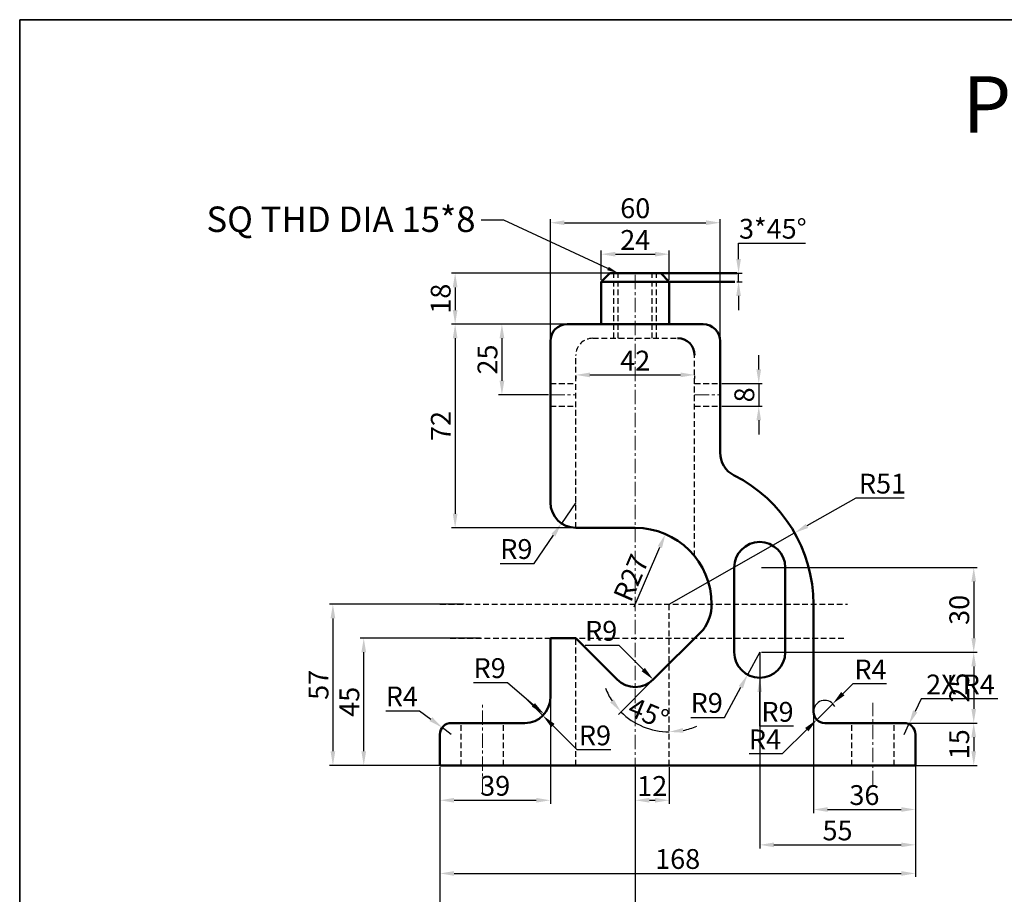
# Model space of a CAD drawing. Units: millimetres. Extents: x -39 to 854, y -107 to 478.
# Tile 2 of 4: x -39 to 309, y 169 to 478. Entities that reach past the tile are written whole.
import ezdxf
from ezdxf import colors
from ezdxf.entities.mleader import LeaderData, LeaderLine
from ezdxf.math import Vec2, Vec3

# ---------------------------------------------------------------- set-up
doc = ezdxf.new("R2010")
doc.units = ezdxf.units.MM
doc.header["$LTSCALE"] = 0.4
doc.linetypes.add('CENTER', pattern=[50.8, 31.75, -6.35, 6.35, -6.35])
doc.linetypes.add('DASHED', pattern=[19.05, 12.7, -6.35])
for name, color, linetype, lineweight in [('M-CNTR', 1, 'CENTER', 18), ('M-DIMS', 2, 'Continuous', 25), ('M-HIDN', 6, 'DASHED', 25), ('M-OUTL', 7, 'Continuous', 50), ('M-TEXT', 3, 'Continuous', 25), ('M-TTLB', 7, 'Continuous', 35)]:
    doc.layers.add(name, color=color, linetype=linetype, lineweight=lineweight)
doc.styles.get("Standard").update_dxf_attribs({"font": 'arial.ttf'})
doc.dimstyles.new('ISO-25', dxfattribs={"dimtxt": 7, "dimasz": 5, "dimexe": 1.25, "dimexo": 0.625, "dimtad": 1, "dimtoh": 1, "dimtxsty": 'Standard', "dimcen": 2.5, "dimadec": 0, "dimazin": 0, "dimtfac": 1, "dimtmove": 0, "dimatfit": 3, "dimfxl": 1, "dimarcsym": 0})

# ---------------------------------------------------------------- blocks, each defined once
blk = doc.blocks.new('*D14')
at = {"layer": 'Defpoints', "color": 0, "ltscale": 0.4, "transparency": 16777216}
for p in [(109.61, 214.19), (277.61, 214.19), (277.61, 176.03)]:
    blk.add_point(p, dxfattribs=at)
at = {"layer": 'M-DIMS', "color": 0, "lineweight": -2, "ltscale": 0.4, "transparency": 16777216}
for p, q in [((109.61, 213.56), (109.61, 174.78)), ((277.61, 213.56), (277.61, 174.78)), ((114.61, 176.03), (272.61, 176.03))]:
    blk.add_line(p, q, dxfattribs=at)
at = {"layer": 'M-DIMS', "color": 0, "ltscale": 0.4, "transparency": 16777216}
for points in [[(114.61, 176.86), (114.61, 175.2), (109.61, 176.03)], [(272.61, 176.86), (272.61, 175.2), (277.61, 176.03)]]:
    blk.add_solid(points, dxfattribs=at)
at = {"layer": 'M-DIMS', "color": 0, "ltscale": 0.4, "transparency": 16777216, "insert": (193.61, 180.23), "char_height": 7, "attachment_point": 5}
blk.add_mtext('168', dxfattribs=at)
blk = doc.blocks.new('*D15')
at = {"layer": 'Defpoints', "color": 0, "ltscale": 0.4, "transparency": 16777216}
for p in [(148.61, 238.19), (109.61, 214.19), (148.61, 201.89)]:
    blk.add_point(p, dxfattribs=at)
at = {"layer": 'M-DIMS', "color": 0, "lineweight": -2, "ltscale": 0.4, "transparency": 16777216}
for p, q in [((148.61, 237.56), (148.61, 200.64)), ((109.61, 213.56), (109.61, 200.64)), ((114.61, 201.89), (143.61, 201.89))]:
    blk.add_line(p, q, dxfattribs=at)
at = {"layer": 'M-DIMS', "color": 0, "ltscale": 0.4, "transparency": 16777216}
for points in [[(114.61, 202.73), (114.61, 201.06), (109.61, 201.89)], [(143.61, 202.73), (143.61, 201.06), (148.61, 201.89)]]:
    blk.add_solid(points, dxfattribs=at)
at = {"layer": 'M-DIMS', "color": 0, "ltscale": 0.4, "transparency": 16777216, "insert": (129.11, 206.1), "char_height": 7, "attachment_point": 5}
blk.add_mtext('39', dxfattribs=at)
blk = doc.blocks.new('*D16')
at = {"layer": 'Defpoints', "color": 0, "ltscale": 0.4, "transparency": 16777216}
for p in [(190.61, 214.19), (178.61, 207.01), (190.61, 201.89)]:
    blk.add_point(p, dxfattribs=at)
at = {"layer": 'M-DIMS', "color": 0, "lineweight": -2, "ltscale": 0.4, "transparency": 16777216}
for p, q in [((190.61, 213.56), (190.61, 200.64)), ((178.61, 206.38), (178.61, 200.64)), ((183.61, 201.89), (185.61, 201.89))]:
    blk.add_line(p, q, dxfattribs=at)
at = {"layer": 'M-DIMS', "color": 0, "ltscale": 0.4, "transparency": 16777216}
for points in [[(183.61, 202.73), (183.61, 201.06), (178.61, 201.89)], [(185.61, 202.73), (185.61, 201.06), (190.61, 201.89)]]:
    blk.add_solid(points, dxfattribs=at)
at = {"layer": 'M-DIMS', "color": 0, "ltscale": 0.4, "transparency": 16777216, "insert": (184.61, 206.03), "char_height": 7, "attachment_point": 5}
blk.add_mtext('12', dxfattribs=at)
blk = doc.blocks.new('*D17')
at = {"layer": 'Defpoints', "color": 0, "ltscale": 0.4, "transparency": 16777216}
for p in [(222.61, 254.19), (277.61, 200.76), (277.61, 186.13)]:
    blk.add_point(p, dxfattribs=at)
at = {"layer": 'M-DIMS', "color": 0, "lineweight": -2, "ltscale": 0.4, "transparency": 16777216}
for p, q in [((222.61, 253.56), (222.61, 184.88)), ((277.61, 200.14), (277.61, 184.88)), ((227.61, 186.13), (272.61, 186.13))]:
    blk.add_line(p, q, dxfattribs=at)
at = {"layer": 'M-DIMS', "color": 0, "ltscale": 0.4, "transparency": 16777216}
for points in [[(227.61, 186.96), (227.61, 185.3), (222.61, 186.13)], [(272.61, 186.96), (272.61, 185.3), (277.61, 186.13)]]:
    blk.add_solid(points, dxfattribs=at)
at = {"layer": 'M-DIMS', "color": 0, "ltscale": 0.4, "transparency": 16777216, "insert": (250.11, 190.32), "char_height": 7, "attachment_point": 5}
blk.add_mtext('55', dxfattribs=at)
blk = doc.blocks.new('*D18')
at = {"layer": 'Defpoints', "color": 0, "ltscale": 0.4, "transparency": 16777216}
for p in [(241.61, 238.74), (277.61, 219.69), (277.61, 198.62)]:
    blk.add_point(p, dxfattribs=at)
at = {"layer": 'M-DIMS', "color": 0, "lineweight": -2, "ltscale": 0.4, "transparency": 16777216}
for p, q in [((241.61, 238.11), (241.61, 197.37)), ((277.61, 219.06), (277.61, 197.37)), ((246.61, 198.62), (272.61, 198.62))]:
    blk.add_line(p, q, dxfattribs=at)
at = {"layer": 'M-DIMS', "color": 0, "ltscale": 0.4, "transparency": 16777216}
for points in [[(246.61, 199.45), (246.61, 197.79), (241.61, 198.62)], [(272.61, 199.45), (272.61, 197.79), (277.61, 198.62)]]:
    blk.add_solid(points, dxfattribs=at)
at = {"layer": 'M-DIMS', "color": 0, "ltscale": 0.4, "transparency": 16777216, "insert": (259.61, 202.82), "char_height": 7, "attachment_point": 5}
blk.add_mtext('36', dxfattribs=at)
blk = doc.blocks.new('*D19')
at = {"layer": 'Defpoints', "color": 0, "ltscale": 0.4, "transparency": 16777216}
for p in [(270.11, 229.19), (270.11, 214.19), (298.24, 214.19)]:
    blk.add_point(p, dxfattribs=at)
at = {"layer": 'M-DIMS', "color": 0, "lineweight": -2, "ltscale": 0.4, "transparency": 16777216}
for p, q in [((270.73, 229.19), (299.49, 229.19)), ((298.24, 224.19), (298.24, 219.19)), ((270.73, 214.19), (299.49, 214.19))]:
    blk.add_line(p, q, dxfattribs=at)
at = {"layer": 'M-DIMS', "color": 0, "ltscale": 0.4, "transparency": 16777216}
for points in [[(297.41, 224.19), (299.07, 224.19), (298.24, 229.19)], [(297.41, 219.19), (299.07, 219.19), (298.24, 214.19)]]:
    blk.add_solid(points, dxfattribs=at)
at = {"layer": 'M-DIMS', "color": 0, "ltscale": 0.4, "transparency": 16777216, "insert": (294.04, 221.69), "char_height": 7, "attachment_point": 5, "rotation": 90}
blk.add_mtext('15', dxfattribs=at)
blk = doc.blocks.new('*D20')
at = {"layer": 'Defpoints', "color": 0, "ltscale": 0.4, "transparency": 16777216}
for p in [(222.61, 254.19), (270.11, 229.19), (298.24, 229.19)]:
    blk.add_point(p, dxfattribs=at)
at = {"layer": 'M-DIMS', "color": 0, "lineweight": -2, "ltscale": 0.4, "transparency": 16777216}
for p, q in [((223.23, 254.19), (299.49, 254.19)), ((298.24, 249.19), (298.24, 234.19)), ((270.73, 229.19), (299.49, 229.19))]:
    blk.add_line(p, q, dxfattribs=at)
at = {"layer": 'M-DIMS', "color": 0, "ltscale": 0.4, "transparency": 16777216}
for points in [[(297.41, 249.19), (299.07, 249.19), (298.24, 254.19)], [(297.41, 234.19), (299.07, 234.19), (298.24, 229.19)]]:
    blk.add_solid(points, dxfattribs=at)
at = {"layer": 'M-DIMS', "color": 0, "ltscale": 0.4, "transparency": 16777216, "insert": (294.04, 241.69), "char_height": 7, "attachment_point": 5, "rotation": 90}
blk.add_mtext('25', dxfattribs=at)
blk = doc.blocks.new('*D21')
at = {"layer": 'Defpoints', "color": 0, "ltscale": 0.4, "transparency": 16777216}
for p in [(222.61, 284.19), (261.36, 254.19), (298.24, 254.19)]:
    blk.add_point(p, dxfattribs=at)
at = {"layer": 'M-DIMS', "color": 0, "lineweight": -2, "ltscale": 0.4, "transparency": 16777216}
for p, q in [((223.23, 284.19), (299.49, 284.19)), ((298.24, 279.19), (298.24, 259.19)), ((261.99, 254.19), (299.49, 254.19))]:
    blk.add_line(p, q, dxfattribs=at)
at = {"layer": 'M-DIMS', "color": 0, "ltscale": 0.4, "transparency": 16777216}
for points in [[(297.41, 279.19), (299.07, 279.19), (298.24, 284.19)], [(297.41, 259.19), (299.07, 259.19), (298.24, 254.19)]]:
    blk.add_solid(points, dxfattribs=at)
at = {"layer": 'M-DIMS', "color": 0, "ltscale": 0.4, "transparency": 16777216, "insert": (294.04, 269.19), "char_height": 7, "attachment_point": 5, "rotation": 90}
blk.add_mtext('30', dxfattribs=at)
blk = doc.blocks.new('*D22')
at = {"layer": 'Defpoints', "color": 0, "ltscale": 0.4, "transparency": 16777216}
for p in [(234.94, 296.4), (190.61, 271.19)]:
    blk.add_point(p, dxfattribs=at)
at = {"layer": 'M-DIMS', "color": 0, "lineweight": -2, "ltscale": 0.4, "transparency": 16777216}
for p, q in [((256.59, 308.71), (239.29, 298.87)), ((273.69, 308.71), (256.59, 308.71)), ((190.61, 271.19), (234.94, 296.4))]:
    blk.add_line(p, q, dxfattribs=at)
at = {"layer": 'M-DIMS', "color": 0, "ltscale": 0.4, "transparency": 16777216}
blk.add_solid([(238.87, 299.59), (239.7, 298.15), (234.94, 296.4)], dxfattribs=at)
at = {"layer": 'M-DIMS', "color": 0, "ltscale": 0.4, "transparency": 16777216, "insert": (266, 312.91), "char_height": 7, "attachment_point": 5}
blk.add_mtext('R51', dxfattribs=at)
blk = doc.blocks.new('*D23')
at = {"layer": 'Defpoints', "color": 0, "ltscale": 0.4, "transparency": 16777216}
for p in [(222.61, 254.19), (218.32, 246.28)]:
    blk.add_point(p, dxfattribs=at)
at = {"layer": 'M-DIMS', "color": 0, "lineweight": -2, "ltscale": 0.4, "transparency": 16777216}
for p, q in [((222.61, 254.19), (218.32, 246.28)), ((210.14, 231.2), (215.93, 241.88)), ((198.22, 231.2), (210.14, 231.2))]:
    blk.add_line(p, q, dxfattribs=at)
at = {"layer": 'M-DIMS', "color": 0, "ltscale": 0.4, "transparency": 16777216}
blk.add_solid([(215.2, 242.28), (216.67, 241.48), (218.32, 246.28)], dxfattribs=at)
at = {"layer": 'M-DIMS', "color": 0, "ltscale": 0.4, "transparency": 16777216, "insert": (203.87, 235.4), "char_height": 7, "attachment_point": 5}
blk.add_mtext('R9', dxfattribs=at)
blk = doc.blocks.new('*D24')
at = {"layer": 'Defpoints', "color": 0, "ltscale": 0.4, "transparency": 16777216}
for p in [(110.4, 227.58), (113.61, 225.19)]:
    blk.add_point(p, dxfattribs=at)
at = {"layer": 'M-DIMS', "color": 0, "lineweight": -2, "ltscale": 0.4, "transparency": 16777216}
for p, q in [((90.5, 233.56), (102.39, 233.56)), ((102.39, 233.56), (106.4, 230.57)), ((113.61, 225.19), (110.4, 227.58))]:
    blk.add_line(p, q, dxfattribs=at)
at = {"layer": 'M-DIMS', "color": 0, "ltscale": 0.4, "transparency": 16777216}
blk.add_solid([(106.89, 231.24), (105.9, 229.9), (110.4, 227.58)], dxfattribs=at)
at = {"layer": 'M-DIMS', "color": 0, "ltscale": 0.4, "transparency": 16777216, "insert": (96.13, 237.69), "char_height": 7, "attachment_point": 5}
blk.add_mtext('R4', dxfattribs=at)
blk = doc.blocks.new('*D25')
at = {"layer": 'Defpoints', "color": 0, "ltscale": 0.4, "transparency": 16777216}
for p in [(157.61, 307.19), (152.53, 299.75)]:
    blk.add_point(p, dxfattribs=at)
at = {"layer": 'M-DIMS', "color": 0, "lineweight": -2, "ltscale": 0.4, "transparency": 16777216}
for p, q in [((157.61, 307.19), (152.53, 299.75)), ((142.86, 285.59), (149.71, 295.63)), ((130.93, 285.59), (142.86, 285.59))]:
    blk.add_line(p, q, dxfattribs=at)
at = {"layer": 'M-DIMS', "color": 0, "ltscale": 0.4, "transparency": 16777216}
blk.add_solid([(149.02, 296.1), (150.4, 295.16), (152.53, 299.75)], dxfattribs=at)
at = {"layer": 'M-DIMS', "color": 0, "ltscale": 0.4, "transparency": 16777216, "insert": (136.59, 289.79), "char_height": 7, "attachment_point": 5}
blk.add_mtext('R9', dxfattribs=at)
blk = doc.blocks.new('*D26')
at = {"layer": 'Defpoints', "color": 0, "ltscale": 0.4, "transparency": 16777216}
for p in [(118.77, 271.19), (71.76, 214.19), (117.11, 214.19)]:
    blk.add_point(p, dxfattribs=at)
at = {"layer": 'M-DIMS', "color": 0, "lineweight": -2, "ltscale": 0.4, "transparency": 16777216}
for p, q in [((118.14, 271.19), (70.51, 271.19)), ((71.76, 266.19), (71.76, 219.19)), ((116.48, 214.19), (70.51, 214.19))]:
    blk.add_line(p, q, dxfattribs=at)
at = {"layer": 'M-DIMS', "color": 0, "ltscale": 0.4, "transparency": 16777216}
for points in [[(70.93, 266.19), (72.6, 266.19), (71.76, 271.19)], [(70.93, 219.19), (72.6, 219.19), (71.76, 214.19)]]:
    blk.add_solid(points, dxfattribs=at)
at = {"layer": 'M-DIMS', "color": 0, "ltscale": 0.4, "transparency": 16777216, "insert": (67.58, 242.69), "char_height": 7, "attachment_point": 5, "rotation": 90}
blk.add_mtext('57', dxfattribs=at)
blk = doc.blocks.new('*D27')
at = {"layer": 'Defpoints', "color": 0, "ltscale": 0.4, "transparency": 16777216}
for p in [(82.66, 259.19), (124.61, 259.19), (124.61, 214.19)]:
    blk.add_point(p, dxfattribs=at)
at = {"layer": 'M-DIMS', "color": 0, "lineweight": -2, "ltscale": 0.4, "transparency": 16777216}
for p, q in [((123.98, 259.19), (81.41, 259.19)), ((82.66, 219.19), (82.66, 254.19)), ((123.98, 214.19), (81.41, 214.19))]:
    blk.add_line(p, q, dxfattribs=at)
at = {"layer": 'M-DIMS', "color": 0, "ltscale": 0.4, "transparency": 16777216}
for points in [[(81.83, 254.19), (83.5, 254.19), (82.66, 259.19)], [(81.83, 219.19), (83.5, 219.19), (82.66, 214.19)]]:
    blk.add_solid(points, dxfattribs=at)
at = {"layer": 'M-DIMS', "color": 0, "ltscale": 0.4, "transparency": 16777216, "insert": (78.48, 236.69), "char_height": 7, "attachment_point": 5, "rotation": 90}
blk.add_mtext('45', dxfattribs=at)
blk = doc.blocks.new('*D28')
at = {"layer": 'Defpoints', "color": 0, "ltscale": 0.4, "transparency": 16777216}
for p in [(190.61, 271.19), (202.61, 262.19), (184.97, 244.55), (178.55, 229.3), (190.61, 214.19)]:
    blk.add_point(p, dxfattribs=at)
at = {"layer": 'M-DIMS', "color": 0, "lineweight": -2, "ltscale": 0.4, "transparency": 16777216}
blk.add_line((184.53, 244.11), (172.67, 232.25), dxfattribs=at)
for start, end in [(201.2009, 213.1005), (225, 270), (281.8995, 293.7991)]:
    blk.add_arc((190.61, 250.19), 24.12, start, end, dxfattribs=at)
at = {"layer": 'M-DIMS', "color": 0, "ltscale": 0.4, "transparency": 16777216}
for points in [[(171.05, 237.54), (169.76, 236.49), (173.55, 233.13)], [(195.67, 225.76), (195.49, 227.42), (190.61, 226.07)]]:
    blk.add_solid(points, dxfattribs=at)
at = {"layer": 'M-DIMS', "color": 0, "ltscale": 0.4, "transparency": 16777216, "insert": (182.98, 231.77), "char_height": 7, "attachment_point": 5, "rotation": 337.5}
blk.add_mtext('45°', dxfattribs=at)
blk = doc.blocks.new('*D29')
at = {"layer": 'Defpoints', "color": 0, "ltscale": 0.4, "transparency": 16777216}
for p in [(178.61, 250.92), (184.97, 244.55)]:
    blk.add_point(p, dxfattribs=at)
at = {"layer": 'M-DIMS', "color": 0, "lineweight": -2, "ltscale": 0.4, "transparency": 16777216}
for p, q in [((160.92, 256.68), (172.84, 256.68)), ((172.84, 256.68), (181.43, 248.09))]:
    blk.add_line(p, q, dxfattribs=at)
at = {"layer": 'M-DIMS', "color": 0, "ltscale": 0.4, "transparency": 16777216}
blk.add_solid([(182.02, 248.68), (180.85, 247.5), (184.97, 244.55)], dxfattribs=at)
at = {"layer": 'M-DIMS', "color": 0, "ltscale": 0.4, "transparency": 16777216, "insert": (166.57, 260.88), "char_height": 7, "attachment_point": 5}
blk.add_mtext('R9', dxfattribs=at)
blk = doc.blocks.new('*D30')
at = {"layer": 'Defpoints', "color": 0, "ltscale": 0.4, "transparency": 16777216}
for p in [(166.61, 370.19), (114.96, 298.19), (168.11, 298.19)]:
    blk.add_point(p, dxfattribs=at)
at = {"layer": 'M-DIMS', "color": 0, "lineweight": -2, "ltscale": 0.4, "transparency": 16777216}
for p, q in [((165.98, 370.19), (113.71, 370.19)), ((114.96, 365.19), (114.96, 303.19)), ((167.48, 298.19), (113.71, 298.19))]:
    blk.add_line(p, q, dxfattribs=at)
at = {"layer": 'M-DIMS', "color": 0, "ltscale": 0.4, "transparency": 16777216}
for points in [[(114.13, 365.19), (115.8, 365.19), (114.96, 370.19)], [(114.13, 303.19), (115.8, 303.19), (114.96, 298.19)]]:
    blk.add_solid(points, dxfattribs=at)
at = {"layer": 'M-DIMS', "color": 0, "ltscale": 0.4, "transparency": 16777216, "insert": (110.82, 334.19), "char_height": 7, "attachment_point": 5, "rotation": 90}
blk.add_mtext('72', dxfattribs=at)
blk = doc.blocks.new('*D31')
at = {"layer": 'Defpoints', "color": 0, "ltscale": 0.4, "transparency": 16777216}
for p in [(178.61, 388.19), (114.96, 370.19), (178.61, 370.19)]:
    blk.add_point(p, dxfattribs=at)
at = {"layer": 'M-DIMS', "color": 0, "lineweight": -2, "ltscale": 0.4, "transparency": 16777216}
for p, q in [((177.98, 388.19), (113.71, 388.19)), ((114.96, 383.19), (114.96, 375.19)), ((177.98, 370.19), (113.71, 370.19))]:
    blk.add_line(p, q, dxfattribs=at)
at = {"layer": 'M-DIMS', "color": 0, "ltscale": 0.4, "transparency": 16777216}
for points in [[(114.13, 383.19), (115.8, 383.19), (114.96, 388.19)], [(114.13, 375.19), (115.8, 375.19), (114.96, 370.19)]]:
    blk.add_solid(points, dxfattribs=at)
at = {"layer": 'M-DIMS', "color": 0, "ltscale": 0.4, "transparency": 16777216, "insert": (110.76, 379.19), "char_height": 7, "attachment_point": 5, "rotation": 90}
blk.add_mtext('18', dxfattribs=at)
blk = doc.blocks.new('*D32')
at = {"layer": 'Defpoints', "color": 0, "ltscale": 0.4, "transparency": 16777216}
for p in [(139.85, 370.19), (131.5, 345.19), (148.61, 345.19)]:
    blk.add_point(p, dxfattribs=at)
at = {"layer": 'M-DIMS', "color": 0, "lineweight": -2, "ltscale": 0.4, "transparency": 16777216}
for p, q in [((139.22, 370.19), (130.25, 370.19)), ((131.5, 365.19), (131.5, 350.19)), ((147.98, 345.19), (130.25, 345.19))]:
    blk.add_line(p, q, dxfattribs=at)
at = {"layer": 'M-DIMS', "color": 0, "ltscale": 0.4, "transparency": 16777216}
for points in [[(130.67, 365.19), (132.34, 365.19), (131.5, 370.19)], [(130.67, 350.19), (132.34, 350.19), (131.5, 345.19)]]:
    blk.add_solid(points, dxfattribs=at)
at = {"layer": 'M-DIMS', "color": 0, "ltscale": 0.4, "transparency": 16777216, "insert": (127.3, 357.69), "char_height": 7, "attachment_point": 5, "rotation": 90}
blk.add_mtext('25', dxfattribs=at)
blk = doc.blocks.new('*D33')
at = {"layer": 'Defpoints', "color": 0, "ltscale": 0.4, "transparency": 16777216}
for p in [(208.61, 349.19), (208.61, 341.19), (222.27, 341.19)]:
    blk.add_point(p, dxfattribs=at)
at = {"layer": 'M-DIMS', "color": 0, "lineweight": -2, "ltscale": 0.4, "transparency": 16777216}
for p, q in [((222.27, 354.19), (222.27, 359.19)), ((209.23, 349.19), (223.52, 349.19)), ((222.27, 349.19), (222.27, 341.19)), ((209.23, 341.19), (223.52, 341.19)), ((222.27, 336.19), (222.27, 331.19))]:
    blk.add_line(p, q, dxfattribs=at)
at = {"layer": 'M-DIMS', "color": 0, "ltscale": 0.4, "transparency": 16777216}
for points in [[(221.44, 354.19), (223.1, 354.19), (222.27, 349.19)], [(221.44, 336.19), (223.1, 336.19), (222.27, 341.19)]]:
    blk.add_solid(points, dxfattribs=at)
at = {"layer": 'M-DIMS', "color": 0, "ltscale": 0.4, "transparency": 16777216, "insert": (218.07, 345.19), "char_height": 7, "attachment_point": 5, "rotation": 90}
blk.add_mtext('8', dxfattribs=at)
blk = doc.blocks.new('*D34')
at = {"layer": 'Defpoints', "color": 0, "ltscale": 0.4, "transparency": 16777216}
for p in [(208.61, 406.05), (148.61, 364.19), (208.61, 364.19)]:
    blk.add_point(p, dxfattribs=at)
at = {"layer": 'M-DIMS', "color": 0, "lineweight": -2, "ltscale": 0.4, "transparency": 16777216}
for p, q in [((148.61, 364.81), (148.61, 407.3)), ((208.61, 364.81), (208.61, 407.3)), ((153.61, 406.05), (203.61, 406.05))]:
    blk.add_line(p, q, dxfattribs=at)
at = {"layer": 'M-DIMS', "color": 0, "ltscale": 0.4, "transparency": 16777216}
for points in [[(153.61, 406.88), (153.61, 405.21), (148.61, 406.05)], [(203.61, 406.88), (203.61, 405.21), (208.61, 406.05)]]:
    blk.add_solid(points, dxfattribs=at)
at = {"layer": 'M-DIMS', "color": 0, "ltscale": 0.4, "transparency": 16777216, "insert": (178.61, 410.25), "char_height": 7, "attachment_point": 5}
blk.add_mtext('60', dxfattribs=at)
blk = doc.blocks.new('*D35')
at = {"layer": 'Defpoints', "color": 0, "ltscale": 0.4, "transparency": 16777216}
for p in [(190.61, 394.92), (166.61, 385.19), (190.61, 385.19)]:
    blk.add_point(p, dxfattribs=at)
at = {"layer": 'M-DIMS', "color": 0, "lineweight": -2, "ltscale": 0.4, "transparency": 16777216}
for p, q in [((166.61, 385.81), (166.61, 396.17)), ((171.61, 394.92), (185.61, 394.92)), ((190.61, 385.81), (190.61, 396.17))]:
    blk.add_line(p, q, dxfattribs=at)
at = {"layer": 'M-DIMS', "color": 0, "ltscale": 0.4, "transparency": 16777216}
for points in [[(171.61, 395.75), (171.61, 394.08), (166.61, 394.92)], [(185.61, 395.75), (185.61, 394.08), (190.61, 394.92)]]:
    blk.add_solid(points, dxfattribs=at)
at = {"layer": 'M-DIMS', "color": 0, "ltscale": 0.4, "transparency": 16777216, "insert": (178.61, 399.05), "char_height": 7, "attachment_point": 5}
blk.add_mtext('24', dxfattribs=at)
blk = doc.blocks.new('*D36')
at = {"layer": 'Defpoints', "color": 0, "ltscale": 0.4, "transparency": 16777216}
for p in [(157.61, 352.52), (199.61, 352.52), (199.61, 352.25)]:
    blk.add_point(p, dxfattribs=at)
at = {"layer": 'M-DIMS', "color": 0, "lineweight": -2, "ltscale": 0.4, "transparency": 16777216}
for p, q in [((157.61, 351.9), (157.61, 351)), ((162.61, 352.25), (194.61, 352.25)), ((199.61, 351.9), (199.61, 351))]:
    blk.add_line(p, q, dxfattribs=at)
at = {"layer": 'M-DIMS', "color": 0, "ltscale": 0.4, "transparency": 16777216}
for points in [[(162.61, 353.08), (162.61, 351.42), (157.61, 352.25)], [(194.61, 353.08), (194.61, 351.42), (199.61, 352.25)]]:
    blk.add_solid(points, dxfattribs=at)
at = {"layer": 'M-DIMS', "color": 0, "ltscale": 0.4, "transparency": 16777216, "insert": (178.61, 356.39), "char_height": 7, "attachment_point": 5}
blk.add_mtext('42', dxfattribs=at)
blk = doc.blocks.new('*D37')
at = {"layer": 'Defpoints', "color": 0, "ltscale": 0.4, "transparency": 16777216}
for p in [(189.28, 295.99), (178.61, 271.19)]:
    blk.add_point(p, dxfattribs=at)
at = {"layer": 'M-DIMS', "color": 0, "lineweight": -2, "ltscale": 0.4, "transparency": 16777216}
blk.add_line((178.22, 270.29), (187.31, 291.39), dxfattribs=at)
at = {"layer": 'M-DIMS', "color": 0, "ltscale": 0.4, "transparency": 16777216}
blk.add_solid([(186.54, 291.72), (188.07, 291.07), (189.28, 295.99)], dxfattribs=at)
at = {"layer": 'M-DIMS', "color": 0, "ltscale": 0.4, "transparency": 16777216, "insert": (177.97, 280.18), "char_height": 7, "attachment_point": 5, "rotation": 66.7097}
blk.add_mtext('R27', dxfattribs=at)
blk = doc.blocks.new('*D38')
at = {"layer": 'Defpoints', "color": 0, "ltscale": 0.4, "transparency": 16777216}
for p in [(139.61, 238.19), (146.43, 232.32)]:
    blk.add_point(p, dxfattribs=at)
at = {"layer": 'M-DIMS', "color": 0, "lineweight": -2, "ltscale": 0.4, "transparency": 16777216}
for p, q in [((121.5, 243.5), (133.43, 243.5)), ((133.43, 243.5), (142.64, 235.58))]:
    blk.add_line(p, q, dxfattribs=at)
at = {"layer": 'M-DIMS', "color": 0, "ltscale": 0.4, "transparency": 16777216}
blk.add_solid([(143.18, 236.21), (142.1, 234.95), (146.43, 232.32)], dxfattribs=at)
at = {"layer": 'M-DIMS', "color": 0, "ltscale": 0.4, "transparency": 16777216, "insert": (127.15, 247.7), "char_height": 7, "attachment_point": 5}
blk.add_mtext('R9', dxfattribs=at)
blk = doc.blocks.new('*D39')
at = {"layer": 'Defpoints', "color": 0, "ltscale": 0.4, "transparency": 16777216}
for p in [(245.61, 233.19), (248.43, 236.02)]:
    blk.add_point(p, dxfattribs=at)
at = {"layer": 'M-DIMS', "color": 0, "lineweight": -2, "ltscale": 0.4, "transparency": 16777216}
for p, q in [((255.51, 243.09), (251.97, 239.55)), ((267.39, 243.09), (255.51, 243.09)), ((245.61, 233.19), (248.43, 236.02))]:
    blk.add_line(p, q, dxfattribs=at)
blk.add_arc((245.61, 233.19), 4, 27.0951, 171.0475, dxfattribs=at)
at = {"layer": 'M-DIMS', "color": 0, "ltscale": 0.4, "transparency": 16777216}
blk.add_solid([(251.38, 240.14), (252.56, 238.96), (248.43, 236.02)], dxfattribs=at)
at = {"layer": 'M-DIMS', "color": 0, "ltscale": 0.4, "transparency": 16777216, "insert": (261.76, 247.21), "char_height": 7, "attachment_point": 5}
blk.add_mtext('R4', dxfattribs=at)
blk = doc.blocks.new('*D40')
at = {"layer": 'Defpoints', "color": 0, "ltscale": 0.4, "transparency": 16777216}
for p in [(213.85, 388.19), (213.85, 385.19), (215.13, 385.19)]:
    blk.add_point(p, dxfattribs=at)
at = {"layer": 'M-DIMS', "color": 0, "lineweight": -2, "ltscale": 0.4, "transparency": 16777216}
for p, q in [((215.13, 393.19), (215.13, 398.8)), ((215.13, 398.8), (238.73, 398.8)), ((214.48, 388.19), (216.38, 388.19)), ((215.13, 385.19), (215.13, 388.19)), ((214.48, 385.19), (216.38, 385.19)), ((215.13, 380.19), (215.13, 375.19))]:
    blk.add_line(p, q, dxfattribs=at)
at = {"layer": 'M-DIMS', "color": 0, "ltscale": 0.4, "transparency": 16777216}
for points in [[(214.3, 393.19), (215.96, 393.19), (215.13, 388.19)], [(214.3, 380.19), (215.96, 380.19), (215.13, 385.19)]]:
    blk.add_solid(points, dxfattribs=at)
at = {"layer": 'M-DIMS', "color": 0, "ltscale": 0.4, "transparency": 16777216, "insert": (227.24, 403), "char_height": 7, "attachment_point": 5}
blk.add_mtext('3*45%%D', dxfattribs=at)
blk = doc.blocks.new('*D74')
at = {"layer": 'Defpoints', "color": 0, "ltscale": 0.4, "transparency": 16777216}
for p in [(109.61, 214.19), (178.61, 214.19), (178.61, 28.68)]:
    blk.add_point(p, dxfattribs=at)
at = {"layer": 'M-DIMS', "color": 0, "lineweight": -2, "ltscale": 0.4, "transparency": 16777216}
for p, q in [((109.61, 213.56), (109.61, 27.43)), ((178.61, 213.56), (178.61, 27.43)), ((114.61, 28.68), (173.61, 28.68))]:
    blk.add_line(p, q, dxfattribs=at)
at = {"layer": 'M-DIMS', "color": 0, "ltscale": 0.4, "transparency": 16777216}
for points in [[(114.61, 29.51), (114.61, 27.84), (109.61, 28.68)], [(173.61, 29.51), (173.61, 27.84), (178.61, 28.68)]]:
    blk.add_solid(points, dxfattribs=at)
at = {"layer": 'M-DIMS', "color": 0, "ltscale": 0.4, "transparency": 16777216, "insert": (144.11, 32.87), "char_height": 7, "attachment_point": 5}
blk.add_mtext('69', dxfattribs=at)
blk = doc.blocks.new('*D81')
at = {"layer": 'Defpoints', "color": 0, "ltscale": 0.4, "transparency": 16777216}
for p in [(139.61, 238.19), (145.97, 231.83)]:
    blk.add_point(p, dxfattribs=at)
at = {"layer": 'M-DIMS', "color": 0, "lineweight": -2, "ltscale": 0.4, "transparency": 16777216}
for p, q in [((139.61, 238.19), (145.97, 231.83)), ((158.1, 219.71), (149.51, 228.29)), ((170.03, 219.71), (158.1, 219.71))]:
    blk.add_line(p, q, dxfattribs=at)
at = {"layer": 'M-DIMS', "color": 0, "ltscale": 0.4, "transparency": 16777216}
blk.add_solid([(150.1, 228.88), (148.92, 227.7), (145.97, 231.83)], dxfattribs=at)
at = {"layer": 'M-DIMS', "color": 0, "ltscale": 0.4, "transparency": 16777216, "insert": (164.38, 223.91), "char_height": 7, "attachment_point": 5}
blk.add_mtext('R9', dxfattribs=at)
blk = doc.blocks.new('*D82')
at = {"layer": 'Defpoints', "color": 0, "ltscale": 0.4, "transparency": 16777216}
for p in [(222.61, 254.19), (222.61, 245.19)]:
    blk.add_point(p, dxfattribs=at)
at = {"layer": 'M-DIMS', "color": 0, "lineweight": -2, "ltscale": 0.4, "transparency": 16777216}
for p, q in [((222.61, 254.19), (222.61, 245.19)), ((222.62, 228.04), (222.61, 240.19)), ((234.54, 228.04), (222.62, 228.04))]:
    blk.add_line(p, q, dxfattribs=at)
at = {"layer": 'M-DIMS', "color": 0, "ltscale": 0.4, "transparency": 16777216}
blk.add_solid([(223.45, 240.19), (221.78, 240.19), (222.61, 245.19)], dxfattribs=at)
at = {"layer": 'M-DIMS', "color": 0, "ltscale": 0.4, "transparency": 16777216, "insert": (228.89, 232.24), "char_height": 7, "attachment_point": 5}
blk.add_mtext('R9', dxfattribs=at)
blk = doc.blocks.new('*D83')
at = {"layer": 'Defpoints', "color": 0, "ltscale": 0.4, "transparency": 16777216}
for p in [(275.35, 228.79), (273.61, 225.19)]:
    blk.add_point(p, dxfattribs=at)
at = {"layer": 'M-DIMS', "color": 0, "lineweight": -2, "ltscale": 0.4, "transparency": 16777216}
for p, q in [((279.72, 237.78), (277.54, 233.28)), ((306.77, 237.78), (279.72, 237.78)), ((273.61, 225.19), (275.35, 228.79))]:
    blk.add_line(p, q, dxfattribs=at)
at = {"layer": 'M-DIMS', "color": 0, "ltscale": 0.4, "transparency": 16777216}
blk.add_solid([(276.79, 233.65), (278.29, 232.92), (275.35, 228.79)], dxfattribs=at)
at = {"layer": 'M-DIMS', "color": 0, "ltscale": 0.4, "transparency": 16777216, "insert": (293.56, 241.92), "char_height": 7, "attachment_point": 5}
blk.add_mtext('2X R4', dxfattribs=at)
blk = doc.blocks.new('*D84')
at = {"layer": 'Defpoints', "color": 0, "ltscale": 0.4, "transparency": 16777216}
for p in [(245.61, 233.19), (242.77, 230.37)]:
    blk.add_point(p, dxfattribs=at)
at = {"layer": 'M-DIMS', "color": 0, "lineweight": -2, "ltscale": 0.4, "transparency": 16777216}
for p, q in [((245.61, 233.19), (242.77, 230.37)), ((230.71, 218.39), (239.22, 226.85)), ((218.82, 218.39), (230.71, 218.39))]:
    blk.add_line(p, q, dxfattribs=at)
at = {"layer": 'M-DIMS', "color": 0, "ltscale": 0.4, "transparency": 16777216}
blk.add_solid([(238.63, 227.44), (239.81, 226.25), (242.77, 230.37)], dxfattribs=at)
at = {"layer": 'M-DIMS', "color": 0, "ltscale": 0.4, "transparency": 16777216, "insert": (224.45, 222.51), "char_height": 7, "attachment_point": 5}
blk.add_mtext('R4', dxfattribs=at)

msp = doc.modelspace()

# ---------------------------------------------------------------- linework, layer by layer
at = {"layer": 'M-CNTR', "ltscale": 0.4}
for p, q in [((178.606, 49.276), (178.606, 388.187)), ((148.606, 345.187), (157.606, 345.187)), ((199.606, 345.187), (208.606, 345.187)), ((124.606, 204.213), (124.606, 235.612)), ((262.606, 207.218), (262.606, 236.329))]:
    msp.add_line(p, q, dxfattribs=at)
at = {"layer": 'M-HIDN', "ltscale": 0.4}
for p, q in [((171.106, 365.187), (171.106, 388.187)), ((172.606, 365.187), (172.606, 388.187)), ((184.606, 365.187), (184.606, 388.187)), ((186.106, 365.187), (186.106, 388.187)), ((163.606, 365.187), (193.606, 365.187)), ((157.606, 298.187), (157.606, 359.187)), ((199.606, 288.158), (199.606, 359.187)), ((148.606, 349.187), (157.606, 349.187)), ((199.606, 349.187), (208.606, 349.187)), ((148.606, 341.187), (157.606, 341.187)), ((199.606, 341.187), (208.606, 341.187)), ((109.606, 271.187), (253.599, 271.187)), ((190.606, 214.187), (190.606, 271.187)), ((113.155, 259.187), (253.185, 259.187)), ((157.606, 214.187), (157.606, 259.187)), ((117.106, 214.187), (117.106, 229.187)), ((132.106, 214.187), (132.106, 229.187)), ((255.106, 214.187), (255.106, 229.187)), ((270.106, 214.187), (270.106, 229.187))]:
    msp.add_line(p, q, dxfattribs=at)
msp.add_arc((163.606, 359.187), 6, 90, 180, dxfattribs=at)
at = {"layer": 'M-OUTL', "ltscale": 0.4}
for p, q in [((169.606, 388.187), (166.606, 385.187)), ((178.606, 388.187), (169.606, 388.187)), ((178.606, 388.187), (187.606, 388.187)), ((187.606, 388.187), (190.606, 385.187)), ((187.606, 388.187), (214.548, 388.187)), ((166.606, 385.187), (166.606, 370.187)), ((166.606, 385.187), (190.606, 385.187)), ((190.606, 370.187), (190.606, 385.187)), ((190.606, 385.187), (213.855, 385.187)), ((154.606, 370.187), (202.606, 370.187)), ((148.606, 364.187), (148.606, 307.187)), ((208.606, 364.187), (208.606, 324.769)), ((157.606, 298.187), (178.606, 298.187)), ((213.606, 284.187), (213.606, 254.187)), ((231.606, 284.187), (231.606, 254.187)), ((241.606, 233.187), (241.606, 271.187)), ((184.97, 244.551), (202.606, 262.187)), ((148.606, 259.187), (157.606, 259.187)), ((148.606, 238.187), (148.606, 259.187)), ((172.243, 244.551), (157.606, 259.187)), ((139.606, 229.187), (113.606, 229.187)), ((273.606, 229.187), (245.606, 229.187)), ((109.606, 225.187), (109.606, 214.187)), ((277.606, 214.187), (277.606, 225.187)), ((109.606, 214.187), (277.606, 214.187)), ((109.606, 214.187), (178.606, 214.187))]:
    msp.add_line(p, q, dxfattribs=at)
for centre, radius, start, end in [((154.606, 364.187), 6, 90, 180), ((202.606, 364.187), 6, 0, 90), ((193.606, 359.187), 6, 0, 90), ((217.606, 324.769), 9, 180, 243.25632), ((190.606, 271.187), 51, 0, 63.25632), ((157.606, 307.187), 9, 180, 270), ((178.606, 271.187), 27, 0, 90), ((222.606, 284.187), 9, 0, 180), ((190.606, 271.187), 15, 323.1301, 0), ((222.606, 254.187), 9, 180, 0), ((178.606, 250.915), 9, 225, 315), ((139.606, 238.187), 9, 270, 0), ((245.606, 233.187), 4, 180, 270), ((113.606, 225.187), 4, 90, 180), ((273.606, 225.187), 4, 0, 90)]:
    msp.add_arc(centre, radius, start, end, dxfattribs=at)
at = {"layer": 'M-TTLB', "ltscale": 0.4}
msp.add_lwpolyline([(-38.928, 477.809), (854.289, 477.809), (854.289, -107.035), (-38.928, -107.035)], close=True, dxfattribs=at)

# ---------------------------------------------------------------- texts
at = {"layer": 'M-TEXT', "ltscale": 0.4, "insert": (294.238, 457.823), "char_height": 20, "attachment_point": 1}
msp.add_mtext_dynamic_manual_height_columns('PIPE VICE', width=220.27302, gutter_width=12.5, heights=[0], dxfattribs=at)

# ---------------------------------------------------------------- dimensions: what is measured, and where the dimension line sits
at = {"layer": 'M-DIMS', "ltscale": 0.4}
for base, p1, p2, override, picture, middle in [((208.606, 406.047), (148.606, 364.187), (208.606, 364.187), {"dimclrd": 0, "dimclre": 0, "dimclrt": 0}, '*D34', (178.606, 410.246)), ((190.606, 394.915), (166.606, 385.187), (190.606, 385.187), {"dimclrd": 0, "dimclre": 0, "dimclrt": 0}, '*D35', (178.606, 399.055)), ((199.606, 352.25), (157.606, 352.521), (199.606, 352.521), {"dimclrd": 0, "dimclre": 0, "dimclrt": 0}, '*D36', (178.606, 356.389)), ((148.606, 201.894), (109.606, 214.187), (148.606, 238.187), {"dimclrd": 0, "dimclre": 0, "dimclrt": 0}, '*D15', (129.106, 206.096)), ((178.606, 28.676), (109.606, 214.187), (178.606, 214.187), {"dimdec": 0, "dimlfac": 1, "dimrnd": 0, "dimzin": 0, "dimdsep": 46, "dimlunit": 2}, '*D74', (144.106, 32.875)), ((190.606, 201.894), (178.606, 207.007), (190.606, 214.187), {"dimclrd": 0, "dimclre": 0, "dimclrt": 0}, '*D16', (184.606, 206.034))]:
    dim = msp.add_linear_dim(base=base, p1=p1, p2=p2, dimstyle='ISO-25', override=override, dxfattribs=at)
    dim.commit()
    dim.dimension.update_dxf_attribs({"geometry": picture, "text_midpoint": middle})
dim = msp.add_linear_dim(base=(215.129, 385.187), p1=(213.855, 388.187), p2=(213.855, 385.187), angle=90, text='<>*45%%D', dimstyle='ISO-25', override={"dimclrd": 0, "dimclre": 0, "dimclrt": 0}, dxfattribs=at)
dim.commit()
dim.dimension.update_dxf_attribs({"geometry": '*D40', "text_midpoint": (227.24, 398.802), "dimtype": 160})
for base, p1, p2, picture, middle in [((114.962, 370.187), (178.606, 388.187), (178.606, 370.187), '*D31', (110.763, 379.187)), ((114.962, 298.187), (166.606, 370.187), (168.106, 298.187), '*D30', (110.823, 334.187)), ((131.503, 345.187), (139.847, 370.187), (148.606, 345.187), '*D32', (127.304, 357.687)), ((222.271, 341.187), (208.606, 349.187), (208.606, 341.187), '*D33', (218.072, 345.187)), ((298.24, 254.187), (222.606, 284.187), (261.361, 254.187), '*D21', (294.038, 269.187)), ((71.764, 214.187), (118.767, 271.187), (117.106, 214.187), '*D26', (67.579, 242.687)), ((298.24, 229.187), (222.606, 254.187), (270.106, 229.187), '*D20', (294.041, 241.687)), ((298.24, 214.187), (270.106, 229.187), (270.106, 214.187), '*D19', (294.041, 221.687))]:
    dim = msp.add_linear_dim(base=base, p1=p1, p2=p2, angle=90, dimstyle='ISO-25', override={"dimclrd": 0, "dimclre": 0, "dimclrt": 0}, dxfattribs=at)
    dim.commit()
    dim.dimension.update_dxf_attribs({"geometry": picture, "text_midpoint": middle})
for center, mpoint, picture, middle in [((190.606, 271.187), (234.94, 296.398), '*D22', (266, 308.709)), ((178.606, 271.187), (189.282, 295.987), '*D37', (181.774, 278.546)), ((178.606, 250.915), (184.97, 244.551), '*D29', (166.569, 256.677)), ((139.606, 238.187), (146.434, 232.323), '*D38', (127.149, 243.496))]:
    dim = msp.add_radius_dim(center=center, mpoint=mpoint, dimstyle='ISO-25', override={"dimclrd": 0, "dimclre": 0, "dimclrt": 0}, dxfattribs=at)
    dim.commit()
    dim.dimension.update_dxf_attribs({"geometry": picture, "text_midpoint": middle, "dimtype": 164})
for center, mpoint, override, picture, middle in [((157.606, 307.187), (152.531, 299.755), {"dimclrd": 0, "dimclre": 0, "dimclrt": 0}, '*D25', (136.586, 289.792)), ((222.606, 254.187), (218.317, 246.275), {"dimclrd": 0, "dimclre": 0, "dimclrt": 0}, '*D23', (203.869, 235.399)), ((222.606, 254.187), (222.61, 245.187), {"dimdec": 0, "dimlfac": 1, "dimrnd": 0, "dimzin": 0, "dimdsep": 46, "dimlunit": 2}, '*D82', (228.893, 232.238)), ((245.606, 233.187), (248.435, 236.016), {"dimclrd": 0, "dimclre": 0, "dimclrt": 0}, '*D39', (261.761, 247.212)), ((113.606, 225.187), (110.401, 227.581), {"dimclrd": 0, "dimclre": 0, "dimclrt": 0}, '*D24', (96.134, 237.689)), ((139.606, 238.187), (145.973, 231.826), {"dimdec": 0, "dimlfac": 1, "dimrnd": 0, "dimzin": 0, "dimdsep": 46, "dimlunit": 2}, '*D81', (164.381, 223.906)), ((245.606, 233.187), (242.768, 230.369), {"dimdec": 0, "dimlfac": 1, "dimrnd": 0, "dimzin": 0, "dimdsep": 46, "dimlunit": 2}, '*D84', (224.452, 222.514))]:
    dim = msp.add_radius_dim(center=center, mpoint=mpoint, dimstyle='ISO-25', override=override, dxfattribs=at)
    dim.commit()
    dim.dimension.update_dxf_attribs({"geometry": picture, "text_midpoint": middle})
dim = msp.add_angular_dim_2l(base=(178.547, 229.3), line1=((190.606, 214.187), (190.606, 271.187)), line2=((184.97, 244.551), (202.606, 262.187)), dimstyle='ISO-25', override={"dimclrd": 0, "dimclre": 0, "dimclrt": 0}, dxfattribs=at)
dim.commit()
dim.dimension.update_dxf_attribs({"geometry": '*D28', "text_midpoint": (182.978, 231.771)})
dim = msp.add_linear_dim(base=(82.663, 259.187), p1=(124.606, 214.187), p2=(124.606, 259.187), angle=90, dimstyle='ISO-25', override={"dimclrd": 0, "dimclre": 0, "dimclrt": 0}, dxfattribs=at)
dim.commit()
dim.dimension.update_dxf_attribs({"geometry": '*D27', "text_midpoint": (82.663, 236.687), "dimtype": 160})
for base, p1, p2, picture, middle in [((277.606, 186.13), (222.606, 254.187), (277.606, 200.761), '*D17', (250.106, 186.13)), ((277.606, 198.618), (241.606, 238.739), (277.606, 219.687), '*D18', (259.606, 198.618)), ((277.606, 176.03), (109.606, 214.187), (277.606, 214.187), '*D14', (193.606, 176.03))]:
    dim = msp.add_linear_dim(base=base, p1=p1, p2=p2, dimstyle='ISO-25', override={"dimclrd": 0, "dimclre": 0, "dimclrt": 0}, dxfattribs=at)
    dim.commit()
    dim.dimension.update_dxf_attribs({"geometry": picture, "text_midpoint": middle, "dimtype": 160})
dim = msp.add_radius_dim(center=(273.606, 225.187), mpoint=(275.354, 228.785), text='2X <>', dimstyle='ISO-25', override={"dimdec": 0, "dimlfac": 1, "dimrnd": 0, "dimzin": 0, "dimdsep": 46, "dimlunit": 2}, dxfattribs=at)
dim.commit()
dim.dimension.update_dxf_attribs({"geometry": '*D83', "text_midpoint": (293.559, 241.922)})

# ---------------------------------------------------------------- leaders
at = {"layer": 'M-TEXT', "ltscale": 0.4}
ml = msp.add_multileader_mtext('Standard', dxfattribs=at)
ml.set_content('SQ THD DIA 15*8', color=256)
ml.set_leader_properties()
ml.build(insert=Vec2(0, 0))
ctx = ml.context
ctx.base_point, ctx.char_height, ctx.plane_origin = Vec3(19.979, 406.925), 9, Vec3(172.606, 388.187)
ctx.text_align_type = 2
notes = []
notes.append((ctx, [(0, (1, 1, 0), (132.176, 406.925), (-1, 0), 8, [(0, [(172.606, 388.187)], 0, [])])]))
ctx.mtext.insert, ctx.mtext.alignment, ctx.mtext.flow_direction = Vec3(122.176, 411.775), 3, 5
for ctx, leaders in notes:
    for number, flags, end, landing, length, lines in leaders:
        leader = LeaderData()
        leader.index, (leader.has_last_leader_line, leader.has_dogleg_vector, leader.attachment_direction) = number, flags
        leader.last_leader_point, leader.dogleg_vector, leader.dogleg_length = Vec3(end), Vec3(landing), length
        for number, points, colour, breaks in lines:
            line = LeaderLine()
            line.index, line.vertices, line.color, line.breaks = number, Vec3.list(points), colors.encode_raw_color(colour), breaks
            leader.lines.append(line)
        ctx.leaders.append(leader)

doc.saveas('drawing.dxf')
